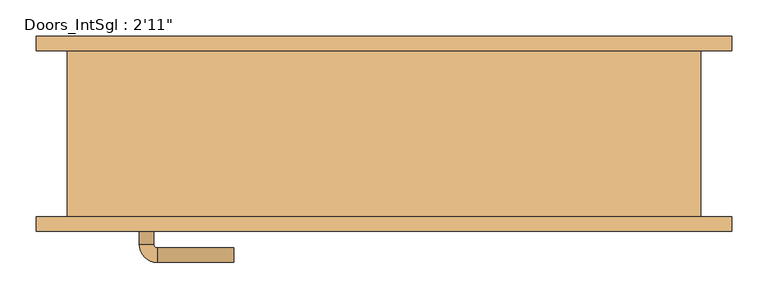
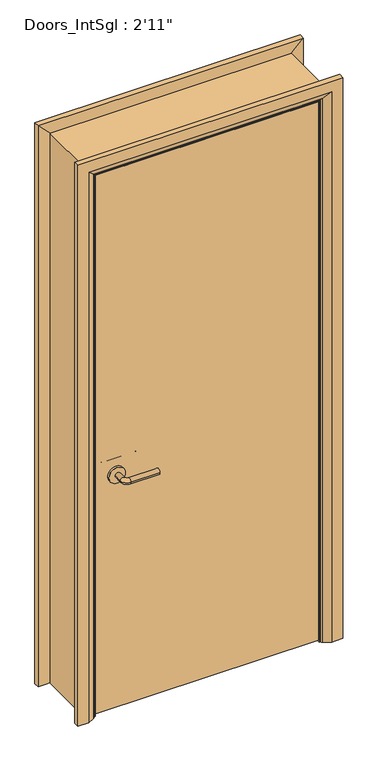
"""IFC4 building model written with IfcOpenShell, lengths in millimetres: door geometry."""

from ifc_helpers import new_model, si_unit, point, frame, frame_2d, origin, place, context, project, spatial, polyline, circle_curve, ellipse_curve, trimmed, segment, composite_curve, outline, extrude, faceted_brep, source, transform, mapped, element, save
from ifc_brep_helpers import plane_surface, cylinder_surface, revolved_surface, advanced_brep


def door_b7cddb0a(model_context):
    return source(origin(), model_context, "Body", "SolidModel", [
        advanced_brep(
        [(-337.5, -68.3, 900.0), (-317.5, -68.3, 900.0), (-337.5, -38.3, 900.0), (-317.5, -38.3, 900.0), (-312.5, -33.3, 900.0), (-312.5, -13.3, 900.0), (-207.5, -13.3, 900.0), (-207.5, -33.3, 900.0)],
        [
            (0, 1, circle_curve(frame((-327.5, -68.3, 900.0), z_axis=(0.0, -1.0, 0.0), x_axis=(1.0, 0.0, 0.0)), 10.0)),
            (1, 0, circle_curve(frame((-327.5, -68.3, 900.0), z_axis=(0.0, -1.0, 0.0), x_axis=(1.0, 0.0, 0.0)), 10.0)),
            (0, 2),
            (2, 3, circle_curve(frame((-327.5, -38.3, 900.0), z_axis=(0.0, -1.0, 0.0), x_axis=(1.0, 0.0, 0.0)), 10.0)),
            (3, 1),
            (3, 2, circle_curve(frame((-327.5, -38.3, 900.0), z_axis=(0.0, -1.0, 0.0), x_axis=(1.0, 0.0, 0.0)), 10.0)),
            (4, 3, circle_curve(frame((-312.5, -38.3, 900.0), z_axis=(0.0, 0.0, 1.0), x_axis=(-1.0, 0.0, 0.0)), 5.0)),
            (2, 5, circle_curve(frame((-312.5, -38.3, 900.0), z_axis=(0.0, 0.0, -1.0), x_axis=(-1.0, 0.0, 0.0)), 25.0)),
            (5, 4, circle_curve(frame((-312.5, -23.3, 900.0), z_axis=(-1.0, 0.0, 0.0), x_axis=(0.0, -1.0, 0.0)), 10.0)),
            (4, 5, circle_curve(frame((-312.5, -23.3, 900.0), z_axis=(-1.0, 0.0, 0.0), x_axis=(0.0, -1.0, 0.0)), 10.0)),
            (6, 7, circle_curve(frame((-207.5, -23.3, 900.0), z_axis=(1.0, 0.0, 0.0), x_axis=(0.0, -1.0, 0.0)), 10.0)),
            (7, 6, circle_curve(frame((-207.5, -23.3, 900.0), z_axis=(1.0, 0.0, 0.0), x_axis=(0.0, -1.0, 0.0)), 10.0)),
            (5, 6),
            (7, 4),
        ],
        [
            plane_surface(frame((-327.5, -68.3, 900.0), z_axis=(0.0, -1.0, 0.0), x_axis=(0.0, 0.0, 1.0))),
            cylinder_surface(frame((-327.5, -68.3, 900.0), z_axis=(0.0, -1.0, 0.0), x_axis=(1.0, 0.0, 0.0)), 10.0),
            revolved_surface(trimmed(ellipse_curve(frame((-327.5, -38.3, 900.0), z_axis=(0.0, -1.0, 0.0), x_axis=(1.0, 0.0, 0.0)), 10.0, 10.0), [point((-337.5, -38.3, 900.0))], [point((-317.5, -38.3, 900.0))], True, "CARTESIAN"), (-312.5, -38.3, 900.0), (0.0, 0.0, -1.0)),
            revolved_surface(trimmed(ellipse_curve(frame((-327.5, -38.3, 900.0), z_axis=(0.0, -1.0, 0.0), x_axis=(1.0, 0.0, 0.0)), 10.0, 10.0), [point((-317.5, -38.3, 900.0))], [point((-337.5, -38.3, 900.0))], True, "CARTESIAN"), (-312.5, -38.3, 900.0), (0.0, 0.0, -1.0)),
            plane_surface(frame((-207.5, -23.3, 900.0), z_axis=(1.0, 0.0, 0.0), x_axis=(0.0, 0.0, 1.0))),
            cylinder_surface(frame((-312.5, -23.3, 900.0), z_axis=(-1.0, 0.0, 0.0), x_axis=(0.0, -1.0, 0.0)), 10.0),
        ],
        [
            (0, [[1, 2]]),
            (1, [[-1, 3, 4, 5]]),
            (1, [[-2, -5, 6, -3]]),
            (2, [[7, -4, 8, 9]]),
            (3, [[-8, -6, -7, 10]]),
            (4, [[11, 12]]),
            (5, [[-9, 13, -12, 14]]),
            (5, [[-10, -14, -11, -13]]),
        ],
    ),
        extrude(outline(composite_curve([segment(trimmed(circle_curve(frame_2d((900.0, -330.0)), 30.0), [point((900.0, -360.0))], [point((900.0, -300.0))], False, "CARTESIAN"), True, "CONTINUOUS"), segment(trimmed(circle_curve(frame_2d((900.0, -330.0)), 30.0), [point((900.0, -300.0))], [point((900.0, -360.0))], False, "CARTESIAN"), True, "CONTINUOUS")], self_intersect=False)), frame((0.0, -76.3, 0.0), z_axis=(0.0, 1.0, 0.0), x_axis=(0.0, 0.0, 1.0)), (0.0, 0.0, 1.0), 8.0),
        advanced_brep(
        [(-337.5, -122.3, 900.0), (-317.5, -122.3, 900.0), (-317.5, -152.3, 900.0), (-337.5, -152.3, 900.0), (-312.5, -157.3, 900.0), (-312.5, -177.3, 900.0), (-207.5, -177.3, 900.0), (-207.5, -157.3, 900.0)],
        [
            (0, 1, circle_curve(frame((-327.5, -122.3, 900.0), z_axis=(0.0, 1.0, 0.0), x_axis=(1.0, 0.0, 0.0)), 10.0)),
            (1, 0, circle_curve(frame((-327.5, -122.3, 900.0), z_axis=(0.0, 1.0, 0.0), x_axis=(1.0, 0.0, 0.0)), 10.0)),
            (1, 2),
            (2, 3, circle_curve(frame((-327.5, -152.3, 900.0), z_axis=(0.0, 1.0, 0.0), x_axis=(1.0, 0.0, 0.0)), 10.0)),
            (3, 0),
            (3, 2, circle_curve(frame((-327.5, -152.3, 900.0), z_axis=(0.0, 1.0, 0.0), x_axis=(1.0, 0.0, 0.0)), 10.0)),
            (4, 5, circle_curve(frame((-312.5, -167.3, 900.0), z_axis=(-1.0, 0.0, 0.0), x_axis=(0.0, 1.0, 0.0)), 10.0)),
            (5, 3, circle_curve(frame((-312.5, -152.3, 900.0), z_axis=(0.0, 0.0, -1.0), x_axis=(-1.0, 0.0, 0.0)), 25.0)),
            (2, 4, circle_curve(frame((-312.5, -152.3, 900.0), z_axis=(0.0, 0.0, 1.0), x_axis=(-1.0, 0.0, 0.0)), 5.0)),
            (5, 4, circle_curve(frame((-312.5, -167.3, 900.0), z_axis=(-1.0, 0.0, 0.0), x_axis=(0.0, 1.0, 0.0)), 10.0)),
            (6, 7, circle_curve(frame((-207.5, -167.3, 900.0), z_axis=(1.0, 0.0, 0.0), x_axis=(0.0, 1.0, 0.0)), 10.0)),
            (7, 6, circle_curve(frame((-207.5, -167.3, 900.0), z_axis=(1.0, 0.0, 0.0), x_axis=(0.0, 1.0, 0.0)), 10.0)),
            (4, 7),
            (6, 5),
        ],
        [
            plane_surface(frame((-327.5, -122.3, 900.0), z_axis=(0.0, 1.0, 0.0), x_axis=(0.0, 0.0, 1.0))),
            cylinder_surface(frame((-327.5, -122.3, 900.0), z_axis=(0.0, 1.0, 0.0), x_axis=(1.0, 0.0, 0.0)), 10.0),
            revolved_surface(trimmed(ellipse_curve(frame((-327.5, -152.3, 900.0), z_axis=(0.0, -1.0, 0.0), x_axis=(1.0, 0.0, 0.0)), 10.0, 10.0), [point((-337.5, -152.3, 900.0))], [point((-317.5, -152.3, 900.0))], True, "CARTESIAN"), (-312.5, -152.3, 900.0), (0.0, 0.0, -1.0)),
            revolved_surface(trimmed(ellipse_curve(frame((-327.5, -152.3, 900.0), z_axis=(0.0, -1.0, 0.0), x_axis=(1.0, 0.0, 0.0)), 10.0, 10.0), [point((-317.5, -152.3, 900.0))], [point((-337.5, -152.3, 900.0))], True, "CARTESIAN"), (-312.5, -152.3, 900.0), (0.0, 0.0, -1.0)),
            plane_surface(frame((-207.5, -167.3, 900.0), z_axis=(1.0, 0.0, 0.0), x_axis=(0.0, 0.0, 1.0))),
            cylinder_surface(frame((-312.5, -167.3, 900.0), z_axis=(-1.0, 0.0, 0.0), x_axis=(0.0, 1.0, 0.0)), 10.0),
        ],
        [
            (0, [[1, 2]]),
            (1, [[3, 4, 5, -2]]),
            (1, [[-5, 6, -3, -1]]),
            (2, [[7, 8, -4, 9]]),
            (3, [[10, -9, -6, -8]]),
            (4, [[11, 12]]),
            (5, [[13, -11, 14, -7]]),
            (5, [[-14, -12, -13, -10]]),
        ],
    ),
        extrude(outline(composite_curve([segment(trimmed(circle_curve(frame_2d((900.0, -330.0)), 30.0), [point((900.0, -360.0))], [point((900.0, -300.0))], False, "CARTESIAN"), True, "CONTINUOUS"), segment(trimmed(circle_curve(frame_2d((900.0, -330.0)), 30.0), [point((900.0, -300.0))], [point((900.0, -360.0))], False, "CARTESIAN"), True, "CONTINUOUS")], self_intersect=False)), frame((0.0, -122.3, 0.0), z_axis=(0.0, 1.0, 0.0), x_axis=(0.0, 0.0, 1.0)), (0.0, 0.0, 1.0), 8.0),
        extrude(outline(polyline([(402.5, -76.3), (402.5, -114.3), (-402.5, -114.3), (-402.5, -76.3), (402.5, -76.3)])), frame((0.0, 0.0, 8.0), z_axis=(0.0, 0.0, 1.0), x_axis=(1.0, 0.0, 0.0)), (0.0, 0.0, 1.0), 2060.0),
        advanced_brep(
        [(479.5, -134.3, 0.0), (439.5, -134.3, 0.0), (413.5, -120.3, 0.0), (409.5, -114.3, 0.0), (479.5, -114.3, 0.0), (479.5, -114.3, 2145.0), (479.5, -134.3, 2145.0), (409.5, -114.3, 2075.0), (-409.5, -114.3, 2075.0), (-409.5, -114.3, 0.0), (-479.5, -114.3, 0.0), (-479.5, -114.3, 2145.0), (413.5, -120.3, 2079.0), (439.5, -134.3, 2105.0), (-479.5, -134.3, 2145.0), (-479.5, -134.3, 0.0), (-439.5, -134.3, 0.0), (-439.5, -134.3, 2105.0), (-413.5, -120.3, 0.0), (-413.5, -120.3, 2079.0)],
        [
            (0, 1),
            (1, 2),
            (2, 3, circle_curve(frame((417.5, -113.3, 0.0), z_axis=(0.0, 0.0, -1.0), x_axis=(1.0, 0.0, 0.0)), 8.0622577)),
            (3, 4),
            (4, 0),
            (4, 5),
            (5, 6),
            (6, 0),
            (3, 7),
            (7, 8),
            (8, 9),
            (9, 10),
            (10, 11),
            (11, 5),
            (2, 12),
            (12, 7, ellipse_curve(frame((417.5, -113.3, 2083.0), z_axis=(0.7071067811865475, 0.0, -0.7071067811865475), x_axis=(-0.7071067811865474, 0.0, -0.7071067811865476)), 11.4017543, 8.0622577)),
            (1, 13),
            (13, 12),
            (6, 14),
            (14, 15),
            (15, 16),
            (16, 17),
            (17, 13),
            (10, 15),
            (14, 11),
            (9, 18, circle_curve(frame((-417.5, -113.3, 0.0), z_axis=(0.0, 0.0, -1.0), x_axis=(-1.0, 0.0, 0.0)), 8.0622577)),
            (18, 16),
            (19, 18),
            (8, 19, ellipse_curve(frame((-417.5, -113.3, 2083.0), z_axis=(-0.7071067811865475, 0.0, -0.7071067811865475), x_axis=(-0.7071067811865474, 0.0, 0.7071067811865476)), 11.4017543, 8.0622577)),
            (19, 17),
            (12, 19),
        ],
        [
            plane_surface(frame((409.5, -114.3, 0.0), z_axis=(0.0, 0.0, -1.0), x_axis=(0.0, 1.0, 0.0))),
            plane_surface(frame((479.5, -134.3, 0.0), z_axis=(1.0, 0.0, 0.0), x_axis=(0.0, 0.0, 1.0))),
            plane_surface(frame((479.5, -114.3, 0.0), z_axis=(0.0, 1.0, 0.0), x_axis=(0.0, 0.0, 1.0))),
            cylinder_surface(frame((417.5, -113.3, 0.0), z_axis=(0.0, 0.0, -1.0), x_axis=(1.0, 0.0, 0.0)), 8.0622577),
            plane_surface(frame((413.5, -120.3, 0.0), z_axis=(-0.4740998230350126, -0.880471099922178, 0.0), x_axis=(0.0, 0.0, 1.0))),
            plane_surface(frame((439.5, -134.3, 0.0), z_axis=(0.0, -1.0, 0.0), x_axis=(0.0, 0.0, 1.0))),
            plane_surface(frame((-479.5, -134.3, 2145.0), z_axis=(-1.0, 0.0, 0.0), x_axis=(0.0, 0.0, -1.0))),
            plane_surface(frame((-409.5, -114.3, 0.0), z_axis=(0.0, 0.0, -1.0), x_axis=(0.0, 1.0, 0.0))),
            cylinder_surface(frame((-417.5, -113.3, 2075.0), z_axis=(0.0, 0.0, 1.0), x_axis=(-1.0, 0.0, 0.0)), 8.0622577),
            plane_surface(frame((-413.5, -120.3, 2079.0), z_axis=(0.47409982303501824, -0.8804710999221749, 0.0), x_axis=(0.0, 0.0, -1.0))),
            plane_surface(frame((479.5, -134.3, 2145.0), z_axis=(0.0, 0.0, 1.0), x_axis=(-1.0, 0.0, 0.0))),
            cylinder_surface(frame((409.5, -113.3, 2083.0), z_axis=(1.0, 0.0, 0.0), x_axis=(0.0, 0.0, 1.0)), 8.0622577),
            plane_surface(frame((413.5, -120.3, 2079.0), z_axis=(0.0, -0.8804710999221764, -0.4740998230350154), x_axis=(-1.0, 0.0, 0.0))),
        ],
        [
            (0, [[1, 2, 3, 4, 5]]),
            (1, [[6, 7, 8, -5]]),
            (2, [[9, 10, 11, 12, 13, 14, -6, -4]]),
            (3, [[15, 16, -9, -3]]),
            (4, [[17, 18, -15, -2]]),
            (5, [[-8, 19, 20, 21, 22, 23, -17, -1]]),
            (6, [[-13, 24, -20, 25]]),
            (7, [[-24, -12, 26, 27, -21]]),
            (8, [[28, -26, -11, 29]]),
            (9, [[-22, -27, -28, 30]]),
            (10, [[-14, -25, -19, -7]]),
            (11, [[31, -29, -10, -16]]),
            (12, [[-23, -30, -31, -18]]),
        ],
    ),
        extrude(outline(polyline([(0.0, -385.5), (2051.0, -385.5), (2051.0, 385.5), (0.0, 385.5), (0.0, 404.5), (2070.0, 404.5), (2070.0, -404.5), (0.0, -404.5), (0.0, -385.5)])), frame((0.0, -74.3, 0.0), z_axis=(0.0, 1.0, 0.0), x_axis=(0.0, 0.0, 1.0)), (0.0, 0.0, 1.0), 32.0),
        advanced_brep(
        [(-479.5, 134.3, 0.0), (-439.5, 134.3, 0.0), (-413.5, 120.3, 0.0), (-409.5, 114.3, 0.0), (-479.5, 114.3, 0.0), (-479.5, 114.3, 2145.0), (-479.5, 134.3, 2145.0), (-409.5, 114.3, 2075.0), (-413.5, 120.3, 2079.0), (-439.5, 134.3, 2105.0), (479.5, 134.3, 0.0), (479.5, 114.3, 0.0), (409.5, 114.3, 0.0), (413.5, 120.3, 0.0), (439.5, 134.3, 0.0), (479.5, 134.3, 2145.0), (439.5, 134.3, 2105.0), (413.5, 120.3, 2079.0), (409.5, 114.3, 2075.0), (479.5, 114.3, 2145.0)],
        [
            (0, 1),
            (1, 2),
            (2, 3, circle_curve(frame((-417.5, 113.3, 0.0), z_axis=(0.0, 0.0, -1.0), x_axis=(-1.0, 0.0, 0.0)), 8.0622577)),
            (3, 4),
            (4, 0),
            (4, 5),
            (5, 6),
            (6, 0),
            (3, 7),
            (7, 5),
            (2, 8),
            (8, 7, ellipse_curve(frame((-417.5, 113.3, 2083.0), z_axis=(-0.7071067811865475, 0.0, -0.7071067811865475), x_axis=(0.7071067811865474, 0.0, -0.7071067811865476)), 11.4017543, 8.0622577)),
            (1, 9),
            (9, 8),
            (6, 9),
            (10, 11),
            (11, 12),
            (12, 13, circle_curve(frame((417.5, 113.3, 0.0), z_axis=(0.0, 0.0, -1.0), x_axis=(1.0, 0.0, 0.0)), 8.0622577)),
            (13, 14),
            (14, 10),
            (15, 10),
            (14, 16),
            (16, 15),
            (13, 17),
            (17, 16),
            (12, 18),
            (18, 17, ellipse_curve(frame((417.5, 113.3, 2083.0), z_axis=(0.7071067811865475, 0.0, -0.7071067811865475), x_axis=(0.7071067811865474, 0.0, 0.7071067811865476)), 11.4017543, 8.0622577)),
            (11, 19),
            (19, 18),
            (15, 19),
            (5, 19),
            (15, 6),
            (7, 18),
            (8, 17),
            (9, 16),
        ],
        [
            plane_surface(frame((-409.5, 187.1010989, 0.0), z_axis=(0.0, 0.0, -1.0), x_axis=(1.0, 0.0, 0.0))),
            plane_surface(frame((-479.5, 134.3, 0.0), z_axis=(-1.0, 0.0, 0.0), x_axis=(0.0, 0.0, 1.0))),
            plane_surface(frame((-479.5, 114.3, 0.0), z_axis=(0.0, -1.0, 0.0), x_axis=(0.0, 0.0, 1.0))),
            cylinder_surface(frame((-417.5, 113.3, 0.0), z_axis=(0.0, 0.0, -1.0), x_axis=(-1.0, 0.0, 0.0)), 8.0622577),
            plane_surface(frame((-413.5, 120.3, 0.0), z_axis=(0.4740998230350183, 0.8804710999221749, 0.0), x_axis=(0.0, 0.0, 1.0))),
            plane_surface(frame((-439.5, 134.3, 0.0), z_axis=(0.0, 1.0, 0.0), x_axis=(0.0, 0.0, 1.0))),
            plane_surface(frame((409.5, 187.1010989, 0.0), z_axis=(0.0, 0.0, -1.0), x_axis=(-1.0, 0.0, 0.0))),
            plane_surface(frame((439.5, 134.3, 2105.0), z_axis=(0.0, 1.0, 0.0), x_axis=(0.0, 0.0, -1.0))),
            plane_surface(frame((413.5, 120.3, 2079.0), z_axis=(-0.4740998230350183, 0.8804710999221749, 0.0), x_axis=(0.0, 0.0, -1.0))),
            cylinder_surface(frame((417.5, 113.3, 2075.0), z_axis=(0.0, 0.0, 1.0), x_axis=(1.0, 0.0, 0.0)), 8.0622577),
            plane_surface(frame((479.5, 114.3, 2145.0), z_axis=(0.0, -1.0, 0.0), x_axis=(0.0, 0.0, -1.0))),
            plane_surface(frame((479.5, 134.3, 2145.0), z_axis=(1.0, 0.0, 0.0), x_axis=(0.0, 0.0, -1.0))),
            plane_surface(frame((-479.5, 134.3, 2145.0), z_axis=(0.0, 0.0, 1.0), x_axis=(1.0, 0.0, 0.0))),
            plane_surface(frame((-479.5, 114.3, 2145.0), z_axis=(0.0, -1.0, 0.0), x_axis=(1.0, 0.0, 0.0))),
            cylinder_surface(frame((-409.5, 113.3, 2083.0), z_axis=(-1.0, 0.0, 0.0), x_axis=(0.0, 0.0, 1.0)), 8.0622577),
            plane_surface(frame((-413.5, 120.3, 2079.0), z_axis=(0.0, 0.8804710999221749, -0.4740998230350183), x_axis=(1.0, 0.0, 0.0))),
            plane_surface(frame((-439.5, 134.3, 2105.0), z_axis=(0.0, 1.0, 0.0), x_axis=(1.0, 0.0, 0.0))),
        ],
        [
            (0, [[1, 2, 3, 4, 5]]),
            (1, [[6, 7, 8, -5]]),
            (2, [[9, 10, -6, -4]]),
            (3, [[11, 12, -9, -3]]),
            (4, [[13, 14, -11, -2]]),
            (5, [[-8, 15, -13, -1]]),
            (6, [[16, 17, 18, 19, 20]]),
            (7, [[21, -20, 22, 23]]),
            (8, [[-22, -19, 24, 25]]),
            (9, [[-24, -18, 26, 27]]),
            (10, [[-26, -17, 28, 29]]),
            (11, [[-28, -16, -21, 30]]),
            (12, [[31, -30, 32, -7]]),
            (13, [[33, -29, -31, -10]]),
            (14, [[34, -27, -33, -12]]),
            (15, [[35, -25, -34, -14]]),
            (16, [[-32, -23, -35, -15]]),
        ],
    ),
        faceted_brep([(-404.5, -114.3, 0.0), (-436.5, -114.3, 0.0), (-436.5, 114.3, 0.0), (-404.5, 114.3, 0.0), (-404.5, 114.3, 2070.0), (-404.5, -114.3, 2070.0), (-436.5, 114.3, 2102.0), (-436.5, -114.3, 2102.0), (404.5, -114.3, 0.0), (404.5, 114.3, 0.0), (436.5, 114.3, 0.0), (436.5, -114.3, 0.0), (404.5, -114.3, 2070.0), (436.5, -114.3, 2102.0), (436.5, 114.3, 2102.0), (404.5, 114.3, 2070.0)], [[[0, 1, 2, 3]], [[3, 4, 5, 0]], [[2, 6, 4, 3]], [[1, 7, 6, 2]], [[0, 5, 7, 1]], [[8, 9, 10, 11]], [[12, 8, 11, 13]], [[13, 11, 10, 14]], [[14, 10, 9, 15]], [[15, 9, 8, 12]], [[4, 15, 12, 5]], [[6, 14, 15, 4]], [[7, 13, 14, 6]], [[5, 12, 13, 7]]]),
    ])


if __name__ == "__main__":
    model = new_model("IFC4")
    model_context = context("Model", 3, world=origin())
    ifc_project = project(units=[si_unit("LENGTHUNIT", "METRE", prefix="MILLI")], contexts=[model_context])
    site = spatial("IfcSite", under=ifc_project)
    building = spatial("IfcBuilding", under=site)
    placement = place(None, origin())
    door_shape = door_b7cddb0a(model_context)
    element("IfcDoor", 1, ObjectType="Doors_IntSgl : 2'11\"", at=placement, inside=building, context=model_context, shape_type="MappedRepresentation", body=[
        mapped(door_shape, transform((0.0, 0.0, 0.0), x_axis=(1.0, 0.0, 0.0), y_axis=(0.0, 1.0, 0.0), z_axis=(0.0, 0.0, 1.0))),
    ])
    save(model, "model.ifc")

# Revit data of these elements
# Type "Doors_IntSgl : 2'11\""
#   Type Mark = "48"
#   Type Comments = "Internal Single"
#   Operation = "SingleSwingRight"
#   Manufacturer = "Revit"
#   Keynote = "L20"
#   Description = "Internal Single Door"
#   Analytic Construction = "Metal"
#   UnderCut = 0' - 0.31496"
#   Tolerance = 0' - 0.07874"
#   Thickness = 0' - 1.49606"
#   Thermal Resistance (R) = 0.270117 (m²·K)/W
#   Structural Tolerance = 0' - 0.31496"
#   StopDepth = 0' - 1.25984"
#   Stop Thickness = 0' - 0.74803"
#   Rough Width = 2' - 11"
#   Rough Height = 6' - 11.07087"
#   Height to Top Lock Rail = 3' - 3.37008"
#   Heat Transfer Coefficient (U) = 3.7021 W/(m²·K)
#   Handle Z Distance = 2' - 11.43307"
#   Handle X Distance = 0' - 2.95276"
#   Frame Thickness = 0' - 1.25984"
#   Door Panel Width = 2' - 7.69291"
#   Door Panel Thickness = 0' - 1.49606"
#   Door Panel Offset = 0' - 0"
#   Height = 6' - 11.07087"
#   Width = 2' - 11"
#   Door Panel Height = 6' - 9.10236"
#   Architrave Setback = 0' - 0.19685"
#   Vis - Ironmongery = yes
#   Material Ironmongery = Door - Handle
#   Material Frame = Door - Frame/Mullion (1)
#   Material Door = Door - Panel
#   Material Architrave = Door - Architrave
#   Visual Light Transmittance = 0
#   Solar Heat Gain Coefficient = 0
#   Function = (empty or 0)
#   Wall Closure = (empty or 0)
# Element 1 (IfcDoor, "Doors_IntSgl : 2'11\"")
#   Materials on its faces: "Door - Architrave", "Door - Handle", "Door - Frame/Mullion (1)", "Door - Panel"
# Materials
#   "Door - Handle": colour RGB 0 0 0, transparency 0, Keynote = "P21", Cost = 0
#   "Door - Frame/Mullion (1)": class "Wood", colour RGB 212 179 113, transparency 0, Keynote = "L20", Cost = 0
#   "Door - Panel": class "Wood", colour RGB 210 159 95, transparency 0, Keynote = "L20", Cost = 0
#   "Door - Architrave": class "Wood", colour RGB 154 90 5, transparency 0, Keynote = "P20", Cost = 0
